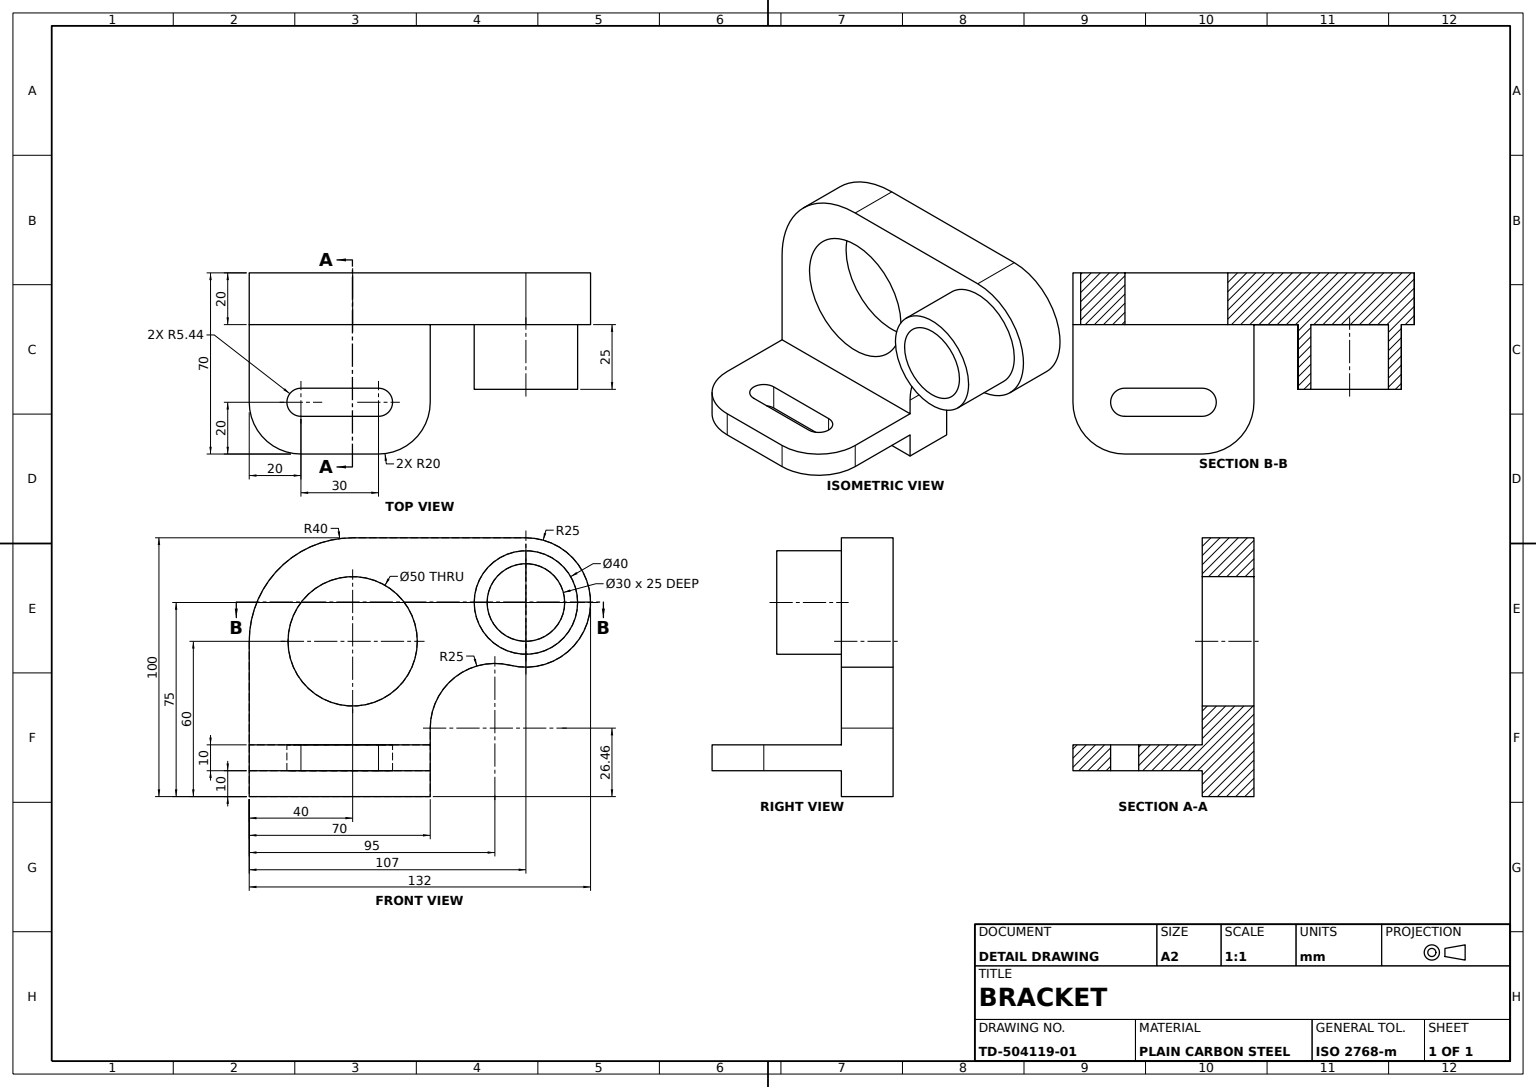
from build123d import *

# Parameters (mm, degrees)
UPRIGHT_PLATE_DEPTH             = 20
BEARING_BOSS_PROFILE_R          = 20
BEARING_BOSS_PROFILE_R_2        = 15
BEARING_BOSS_DEPTH              = 25
BEARING_BORE_SKETCH_R           = 25
BEARING_BORE_50_DEPTH           = 168.478356811
BASE_PLATE_PROFILE_W            = 70
BASE_PLATE_PROFILE_H            = 10
BASE_PLATE_DEPTH                = 50
BASE_PLATE_CORNER_FILLETS_R20_R = 20
MOUNTING_SLOT_DEPTH             = 170.481562419


with BuildPart() as part:
    # Upright Plate Profile → Upright Plate (new body)
    with BuildSketch(Plane.XY):
        with BuildLine():
            Line((0, 0), (70, 0))
            Line((70, 0), (70, 26.461355602))
            ThreePointArc((70, 26.461355602), (79.588964993, 46.146375287), (101, 50.730677801))
            ThreePointArc((101, 50.730677801), (131.816658266, 71.977836452), (107, 100))
            Line((107, 100), (40, 100))
            ThreePointArc((40, 100), (11.715728753, 88.284271247), (0, 60))
            Line((0, 60), (0, 0))
        make_face()
    extrude(amount=UPRIGHT_PLATE_DEPTH)

    # Bearing Boss Profile → Bearing Boss (add)
    with BuildSketch(Plane.XY.offset(20)):
        with Locations(Location((107, 75, 0), (0, 0, 180))):
            Circle(BEARING_BOSS_PROFILE_R)
        with Locations((107, 75)):
            Circle(BEARING_BOSS_PROFILE_R_2, mode=Mode.SUBTRACT)
    extrude(amount=BEARING_BOSS_DEPTH)

    # Bearing Bore Sketch → Bearing Bore Ø50 (cut, through all)
    with BuildSketch(Plane.XY.offset(20)):
        with Locations((40, 60)):
            Circle(BEARING_BORE_SKETCH_R)
    extrude(amount=-BEARING_BORE_50_DEPTH, mode=Mode.SUBTRACT)

    # Base Plate Profile → Base Plate (add)
    with BuildSketch(Plane.XY.offset(20)):
        with Locations((35, 15)):
            Rectangle(BASE_PLATE_PROFILE_W, BASE_PLATE_PROFILE_H)
    extrude(amount=BASE_PLATE_DEPTH)

    # Base Plate Corner Fillets R20
    base_plate_corner_fillets_r20_edges = [part.edges().sort_by_distance(p)[0] for p in [
        (70, 15, 70),
        (0, 15, 70),
    ]]
    fillet(base_plate_corner_fillets_r20_edges, radius=BASE_PLATE_CORNER_FILLETS_R20_R)

    # Mounting Slot Sketch → Mounting Slot (cut, through all)
    with BuildSketch(Plane(origin=(0, 20, 0), x_dir=(1, 0, 0), z_dir=(0, 1, 0))):
        with BuildLine():
            Line((20, -44.564709442), (50, -44.564709442))
            ThreePointArc((50, -44.564709442), (55.435290558, -50), (50, -55.435290558))
            Line((50, -55.435290558), (20, -55.435290558))
            ThreePointArc((20, -55.435290558), (14.564709442, -50), (20, -44.564709442))
        make_face()
    extrude(amount=-MOUNTING_SLOT_DEPTH, mode=Mode.SUBTRACT)


solid = part.part
